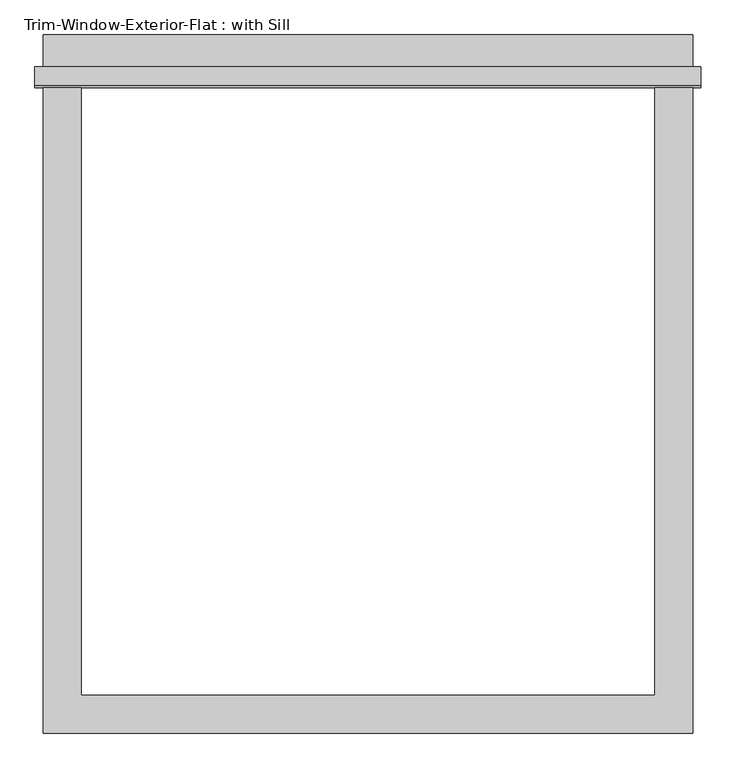
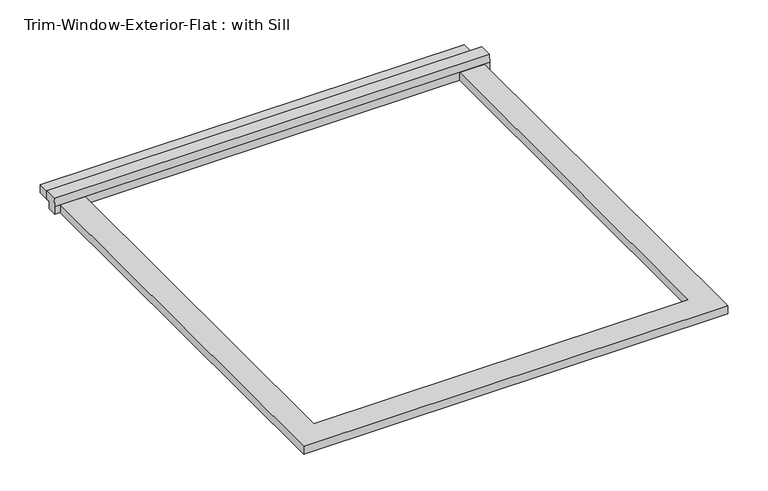
"""IFC4 building model written with IfcOpenShell, lengths in millimetres: proxy geometry, Trim-Window-Exterior-Flat : with Sill."""

from ifc_helpers import new_model, si_unit, frame, origin, origin_with_axes, place, context, project, spatial, polyline, outline, extrude, source, transform, mapped, element, save


def trim_window_exterior_flat_with_sill_f2223f96(model_context):
    return source(origin(), model_context, "Body", "SweptSolid", [
        extrude(outline(polyline([(488.95, 936.5823709), (-488.95, 936.5823709), (-488.95, 993.7323709), (488.95, 993.7323709), (488.95, 936.5823709)])), origin_with_axes(), (0.0, 0.0, 1.0), 19.05),
        extrude(outline(polyline([(946.15, 38.1), (946.15, 19.05), (936.5823709, 19.05), (936.5823709, 0.0), (914.4, 0.0), (914.4, 19.05), (916.8580645, 38.1), (946.15, 38.1)])), frame((-501.65, 0.0, 0.0), z_axis=(1.0, 0.0, 0.0), x_axis=(0.0, 1.0, 0.0)), (0.0, 0.0, 1.0), 1003.3),
        extrude(outline(polyline([(-488.95, -57.15), (-488.95, 914.4), (-431.8, 914.4), (-431.8, 0.0), (431.8, 0.0), (431.8, 914.4), (488.95, 914.4), (488.95, -57.15), (-488.95, -57.15)])), origin_with_axes(), (0.0, 0.0, 1.0), 19.05),
    ])


if __name__ == "__main__":
    model = new_model("IFC4")
    model_context = context("Model", 3, world=origin())
    ifc_project = project(units=[si_unit("LENGTHUNIT", "METRE", prefix="MILLI")], contexts=[model_context])
    site = spatial("IfcSite", under=ifc_project)
    building = spatial("IfcBuilding", under=site)
    placement = place(None, origin())
    trim_window_exterior_flat_with_sill_shape = trim_window_exterior_flat_with_sill_f2223f96(model_context)
    element("IfcBuildingElementProxy", 1, Name="Trim-Window-Exterior-Flat : with Sill", ObjectType="Trim-Window-Exterior-Flat : with Sill", at=placement, inside=building, context=model_context, shape_type="MappedRepresentation", body=[
        mapped(trim_window_exterior_flat_with_sill_shape, transform((0.0, 0.0, 0.0), x_axis=(1.0, 0.0, 0.0), y_axis=(0.0, 1.0, 0.0), z_axis=(0.0, 0.0, 1.0))),
    ])
    save(model, "model.ifc")

# Revit data of these elements
# Type "Trim-Window-Exterior-Flat : with Sill"
#   Trim Width = 0' - 2 1/4"
#   Trim Thickness_Picture Frame = 0' - 1 1/4"
#   Trim Thickness_with Sill = 0' - 0 3/4"
#   Sill Thickness = 0' - 1 1/4"
#   Opening Width [instance default] = 2' - 0"
#   Opening Height [instance default] = 3' - 0"
#   Default Elevation = 4' - 0"
#   Sill = yes
#   Picture Frame = no
#   Trim Material [instance default] = none
# Element 1 (IfcBuildingElementProxy, "Trim-Window-Exterior-Flat : with Sill")
#   Opening Width = 2' - 10"
#   Trim Material = Clad - White
#   Materials on its faces: "Clad - White"
# Materials
#   "Clad - White": class "Wood", colour RGB 242 242 238, transparency 0, Cost = 0
